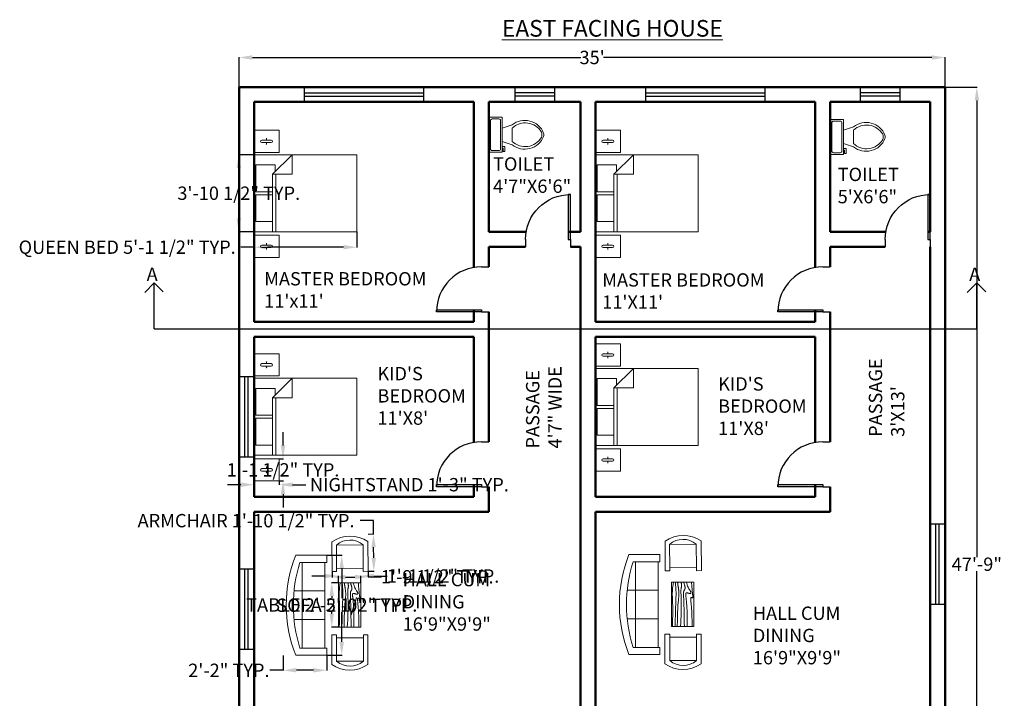
# Model space of a CAD drawing. Units: inches. Extents: x 179 to 2009, y 628 to 2084.
# Tile 4 of 5: x 635 to 1226, y 1676 to 2084. Entities that reach past the tile are written whole.
import ezdxf

# ---------------------------------------------------------------- set-up
doc = ezdxf.new("R2010")
doc.units = ezdxf.units.IN
doc.header["$MEASUREMENT"] = 0
for name, color, linetype, lineweight in [('A-ANNO-DIMS', 2, 'Continuous', 18), ('A-ANNO-SYMB', 5, 'Continuous', 25), ('A-ANNO-TEXT', 7, 'Continuous', 18), ('A-DOOR', 3, 'Continuous', 25), ('A-FURN', 4, 'Continuous', 18), ('A-GLAZ', 2, 'Continuous', 25), ('A-WALL', 1, 'Continuous', 50)]:
    doc.layers.add(name, color=color, linetype=linetype, lineweight=lineweight)
doc.styles.get("Standard").update_dxf_attribs({"font": 'arial.ttf'})
doc.dimstyles.get("Standard").update_dxf_attribs({"dimtxt": 8, "dimasz": 8, "dimexe": 0.18, "dimexo": 0.0625, "dimgap": 0.09, "dimtad": 0, "dimtih": 1, "dimtoh": 1, "dimdec": 0, "dimzin": 0, "dimdsep": 46, "dimlunit": 3, "dimtxsty": 'Standard', "dimcen": 0.09, "dimadec": 0, "dimazin": 0, "dimtfac": 1, "dimtdec": 0, "dimtofl": 0, "dimtmove": 0, "dimatfit": 3, "dimfxl": 1, "dimtolj": 1, "dimtzin": 0, "dimarcsym": 0})

# ---------------------------------------------------------------- blocks, each defined once
blk = doc.blocks.new('*U4')
for p, q in [((0, 0), (0, -6)), ((36, 0), (36, -6))]:
    blk.add_line(p, q)
blk.add_lwpolyline([(0, 0), (0, 36), (1.75, 36), (1.75, 0)], close=True)
blk.add_arc((0, 0), 36, 0, 90)
blk = doc.blocks.new('Bed - Queen')
for p, q in [((0, -80.00003), (0, 0)), ((0, 0), (59.99999, 0)), ((59.99999, 0), (59.99999, -80.00003)), ((7.99999, -1.2), (28.79998, -1.2)), ((7.99999, -14.4), (7.99999, -1.2)), ((28.79998, -1.2), (28.79998, -14.4)), ((31.19999, -1.2), (51.99999, -1.2)), ((31.19999, -14.4), (31.19999, -1.2)), ((51.99999, -1.2), (51.99999, -16.4)), ((0, -14.4), (44.8, -14.4)), ((59.99999, -29.6), (44.8, -14.4)), ((44.8, -14.4), (44.8, -29.6)), ((44.8, -16.8), (0, -16.8)), ((51.99999, -16.4), (46.79936, -16.4)), ((44.8, -29.6), (59.99999, -29.6)), ((59.99999, -80.00003), (0, -80.00003))]:
    blk.add_line(p, q)
blk = doc.blocks.new('*U3')
for p, q in [((9.5, -6), (9.5, -2)), ((-10, -8.5), (-8, -8.5)), ((-10, -9.5), (-10, -8.5)), ((-7, -9.5), (-10, -9.5)), ((-8, -8.5), (-8, -8)), ((-7, -8), (-7, -9.5)), ((-4, -8), (-6, -14)), ((4, -8), (6, -14)), ((4, -14), (-4, -14))]:
    blk.add_line(p, q)
blk.add_lwpolyline([(10.5, -8), (10.5, 0), (-10.5, 0), (-10.5, -8)], close=True)
for points in [[(-9.5, -2), (-9.5, -6)], [(8.5, -1), (-8.5, -1)], [(-8.5, -7), (8.5, -7)]]:
    blk.add_lwpolyline(points)
for centre, radius, start, end in [((-8.62, -1.88), 0.884, 81.8699, 188.1301), ((8.62, -1.88), 0.884, 351.8699, 98.1301), ((-8.62, -6.12), 0.884, 171.8699, 278.1301), ((8.62, -6.12), 0.884, 261.8699, 8.1301), ((3.52, -21.58), 12.17, 141.46911, 247.97143), ((4.2, -21.82), 11.33, 136.36773, 238.94682), ((-3.52, -21.58), 12.17, 292.02843, 38.53071), ((-4.2, -21.82), 11.33, 301.05301, 43.63209), ((0, -27.88), 4, 245.73182, 294.26817), ((0, -29), 4, 254.86053, 285.13947)]:
    blk.add_arc(centre, radius, start, end)
blk = doc.blocks.new('Sofa - Roundback 7 ft.')
for p, q in [((-12.00002, -32.4421), (-12.00003, -6.5971)), ((11.99997, -32.4421), (11.99998, -6.5971)), ((-36.000027, -34), (-36.000027, -11.4696)), ((-35.999844, -13.3819), (35.9998, -13.3819)), ((35.99998, -34), (35.99998, -11.4696)), ((-36.000027, -32.4421), (35.99998, -32.4421))]:
    blk.add_line(p, q)
for points in [[(-36.000027, -34), (-42.000027, -34), (-42.000027, -8)], [(41.99998, -8), (41.99998, -34), (35.99998, -34)]]:
    blk.add_lwpolyline(points)
for centre, radius, start, end in [((0, -114.25), 114.25, 68.43141, 111.5686), ((-0.00001, -127.1968), 121.1968, 72.72033, 107.2797)]:
    blk.add_arc(centre, radius, start, end)
blk = doc.blocks.new('Table - Rectangular Woodgrain 60 x 30 in.')
for p, q in [((0, 0), (0, -30)), ((60, 0), (0, 0)), ((60, -30), (60, 0)), ((0, -30), (60, -30))]:
    blk.add_line(p, q)
for points in [[(0, -2.4), (4.8155, -2.418), (9.0302, -2.4688), (12.709, -2.5477), (15.9167, -2.65), (18.7181, -2.7711), (21.1781, -2.9063), (23.3616, -3.0508), (25.3333, -3.2), (27.1477, -3.3495), (28.8172, -3.4958), (30.3437, -3.636), (31.7291, -3.7667), (32.9756, -3.8849), (34.0849, -3.9875), (35.059, -4.0714), (35.9, -4.1334), (36.6114, -4.1711), (37.2041, -4.1854), (37.6906, -4.1779), (38.0833, -4.15), (38.3948, -4.1034), (38.6375, -4.0396), (38.8239, -3.9602), (38.9666, -3.8667), (39.0764, -3.7608), (39.1573, -3.6448), (39.2116, -3.521), (39.2416, -3.3917), (39.2498, -3.2593), (39.2385, -3.1261), (39.21, -2.9944), (39.1666, -2.8667), (39.111, -2.7447), (39.0468, -2.6281), (38.978, -2.5163), (38.9083, -2.4083), (38.8418, -2.3035), (38.7823, -2.201), (38.7337, -2.1001), (38.7, -2), (38.6844, -1.9003), (38.6875, -1.8021), (38.7094, -1.707), (38.75, -1.6167), (38.8094, -1.5326), (38.8875, -1.4563), (38.9844, -1.3893), (39.1, -1.3333), (39.2351, -1.2896), (39.3937, -1.2583), (39.5804, -1.2396), (39.8, -1.2333), (40.057, -1.2396), (40.3562, -1.2583), (40.7023, -1.2896), (41.1, -1.3333), (41.5547, -1.3895), (42.0755, -1.4573), (42.6721, -1.5361), (43.3542, -1.625), (44.1316, -1.7233), (45.014, -1.8302), (46.0114, -1.9449), (47.1333, -2.0667), (48.3862, -2.1947), (49.7625, -2.3281), (51.2513, -2.4663), (52.8416, -2.6083), (54.5226, -2.7535), (56.2833, -2.9011), (58.1127, -3.0501), (60, -3.2)], [(0, -9.2), (6.5759, -9.0858), (11.9385, -9.0365), (16.2527, -9.0418), (19.6833, -9.0917), (22.3952, -9.1759), (24.5531, -9.2844), (26.322, -9.4069), (27.8666, -9.5333), (29.3241, -9.6553), (30.7203, -9.7719), (32.0532, -9.8837), (33.3208, -9.9917), (34.5213, -10.0965), (35.6526, -10.199), (36.7128, -10.2999), (37.7, -10.4), (38.6129, -10.4996), (39.4531, -10.5969), (40.223, -10.6895), (40.925, -10.775), (41.5613, -10.8512), (42.1344, -10.9156), (42.6465, -10.966), (43.1, -11), (43.4976, -11.0158), (43.8437, -11.0136), (44.143, -10.9942), (44.4, -10.9583), (44.6195, -10.9069), (44.8062, -10.8406), (44.9648, -10.7603), (45.1, -10.6667), (45.2155, -10.5598), (45.3114, -10.4365), (45.3871, -10.2929), (45.4416, -10.125), (45.4743, -9.929), (45.4844, -9.7011), (45.4709, -9.4371), (45.4333, -9.1333), (45.3716, -8.7883), (45.2896, -8.4104), (45.1919, -8.0107), (45.0833, -7.6), (44.9685, -7.1893), (44.8521, -6.7896), (44.7388, -6.4117), (44.6333, -6.0667), (44.54, -5.7628), (44.4614, -5.4979), (44.4001, -5.2675), (44.3583, -5.0667), (44.3384, -4.8909), (44.3427, -4.7354), (44.3736, -4.5956), (44.4333, -4.4667), (44.5236, -4.3453), (44.6427, -4.2333), (44.7884, -4.1339), (44.9583, -4.05), (45.1501, -3.9849), (45.3614, -3.9417), (45.59, -3.9234), (45.8333, -3.9333), (46.0915, -3.9749), (46.3734, -4.0531), (46.6906, -4.1736), (47.0542, -4.3417), (47.4756, -4.5629), (47.9661, -4.8427), (48.5372, -5.1866), (49.2, -5.6), (49.9676, -6.0844), (50.8594, -6.625), (51.8965, -7.2031), (53.1, -7.8), (54.491, -8.3969), (56.0906, -8.975), (57.9199, -9.5156), (60, -10)], [(0, -12.8), (5.1847, -12.9322), (9.6213, -13.0323), (13.3963, -13.1059), (16.5958, -13.1583), (19.3063, -13.1952), (21.614, -13.2219), (23.6054, -13.2439), (25.3666, -13.2667), (26.9728, -13.2947), (28.4531, -13.3281), (29.8256, -13.3663), (31.1083, -13.4083), (32.3191, -13.4535), (33.476, -13.501), (34.597, -13.5501), (35.7, -13.6), (36.7984, -13.6497), (37.8875, -13.6979), (38.9578, -13.743), (40, -13.7833), (41.0047, -13.8174), (41.9625, -13.8438), (42.864, -13.8607), (43.7, -13.8667), (44.4631, -13.8604), (45.1552, -13.8417), (45.7801, -13.8104), (46.3416, -13.7667), (46.8439, -13.7104), (47.2906, -13.6417), (47.6858, -13.5604), (48.0333, -13.4667), (48.3375, -13.3608), (48.6042, -13.2448), (48.8396, -13.121), (49.05, -12.9917), (49.2417, -12.8593), (49.4208, -12.7261), (49.5937, -12.5944), (49.7667, -12.4667), (49.9452, -12.3451), (50.1323, -12.2313), (50.3303, -12.1268), (50.5416, -12.0333), (50.7686, -11.9524), (51.0135, -11.8854), (51.2788, -11.8341), (51.5666, -11.8), (51.8785, -11.7843), (52.2116, -11.7865), (52.562, -11.8059), (52.926, -11.8417), (53.2998, -11.8931), (53.6795, -11.9594), (54.0614, -12.0397), (54.4416, -12.1333), (54.8223, -12.2401), (55.2293, -12.3625), (55.6942, -12.5037), (56.2489, -12.6667), (56.9251, -12.8547), (57.7545, -13.0708), (58.7689, -13.3182), (60, -13.6)], [(0, -18), (5.124, -17.7273), (9.6609, -17.5057), (13.6705, -17.3303), (17.2125, -17.1958), (20.3467, -17.0973), (23.1328, -17.0297), (25.6307, -16.9878), (27.9, -16.9667), (29.9928, -16.9617), (31.9302, -16.9703), (33.7254, -16.9907), (35.3917, -17.0208), (36.9423, -17.0588), (38.3906, -17.1026), (39.7499, -17.1503), (41.0333, -17.2), (42.2519, -17.2496), (43.4073, -17.2969), (44.4986, -17.3395), (45.525, -17.375), (46.4858, -17.4012), (47.3802, -17.4156), (48.2074, -17.416), (48.9667, -17.4), (49.6583, -17.3662), (50.2872, -17.3167), (50.8595, -17.2547), (51.3812, -17.1833), (51.8584, -17.1057), (52.2971, -17.025), (52.7034, -16.9443), (53.0833, -16.8667), (53.443, -16.7951), (53.789, -16.7313), (54.128, -16.6768), (54.4666, -16.6334), (54.8115, -16.6024), (55.1693, -16.5854), (55.5465, -16.5841), (55.95, -16.6), (56.3828, -16.6337), (56.8346, -16.6823), (57.2915, -16.7418), (57.7396, -16.8084), (58.165, -16.878), (58.5539, -16.9469), (58.8924, -17.0111), (59.1666, -17.0667), (59.3679, -17.1107), (59.5078, -17.1438), (59.6032, -17.1675), (59.6708, -17.1833), (59.7275, -17.193), (59.7901, -17.1979), (59.8753, -17.1998), (60, -17.2)], [(0, -22.4), (8.0098, -22.2501), (14.4094, -22.1011), (19.4168, -21.9535), (23.25, -21.8083), (26.1269, -21.6663), (28.2656, -21.5281), (29.884, -21.3947), (31.2, -21.2667), (32.3967, -21.1448), (33.5172, -21.0292), (34.5697, -20.9198), (35.5625, -20.8167), (36.5037, -20.7198), (37.4015, -20.6292), (38.2642, -20.5448), (39.1, -20.4667), (39.9164, -20.3951), (40.7187, -20.3313), (41.5117, -20.2768), (42.3, -20.2333), (43.0883, -20.2024), (43.8812, -20.1854), (44.6836, -20.1841), (45.5, -20.2), (46.3328, -20.234), (47.1747, -20.2844), (48.0163, -20.3488), (48.8479, -20.425), (49.66, -20.5106), (50.4429, -20.6031), (51.1872, -20.7004), (51.8833, -20.8), (52.5246, -20.8999), (53.1166, -20.9995), (53.6681, -21.0983), (54.1875, -21.1958), (54.6834, -21.2919), (55.1646, -21.3859), (55.6394, -21.4777), (56.1167, -21.5667), (56.6028, -21.6515), (57.0961, -21.7266), (57.5929, -21.7852), (58.0896, -21.8208), (58.5823, -21.8268), (59.0674, -21.7964), (59.5412, -21.723), (60, -21.6)], [(0, -25.2), (8.6355, -25.0504), (15.7026, -24.9031), (21.4049, -24.7606), (25.9458, -24.625), (29.529, -24.4988), (32.3578, -24.3844), (34.6359, -24.284), (36.5667, -24.2), (38.3213, -24.1341), (39.9417, -24.0854), (41.437, -24.0523), (42.8167, -24.0333), (44.0901, -24.0268), (45.2667, -24.0313), (46.3557, -24.0451), (47.3667, -24.0667), (48.309, -24.0947), (49.1928, -24.1287), (50.0284, -24.168), (50.826, -24.2125), (51.5959, -24.2617), (52.3483, -24.3151), (53.0935, -24.3725), (53.8417, -24.4334), (54.6009, -24.497), (55.3699, -24.561), (56.1454, -24.6226), (56.9239, -24.6792), (57.7021, -24.7279), (58.4764, -24.7662), (59.2435, -24.7911), (60, -24.8)], [(0, -28.8), (5.6867, -28.6681), (10.45, -28.5698), (14.407, -28.5012), (17.675, -28.4584), (20.3711, -28.4374), (22.6125, -28.4344), (24.5164, -28.4455), (26.2, -28.4667), (27.762, -28.4947), (29.2276, -28.5281), (30.6033, -28.5663), (31.8958, -28.6084), (33.1118, -28.6535), (34.2578, -28.7011), (35.3405, -28.7501), (36.3666, -28.8), (37.3443, -28.8497), (38.288, -28.8974), (39.2137, -28.9412), (40.1375, -28.9792), (41.0753, -29.0093), (42.0432, -29.0297), (43.0572, -29.0384), (44.1333, -29.0333), (45.2936, -29.0114), (46.5843, -28.9641), (48.0579, -28.8816), (49.7666, -28.7542), (51.7629, -28.5721), (54.0989, -28.3255), (56.8272, -28.0048), (60, -27.6)]]:
    blk.add_lwpolyline(points)
blk = doc.blocks.new('*D17')
at = {"layer": 'A-ANNO-DIMS', "color": 0, "lineweight": -2, "transparency": 16777216}
for p, q in [((766.49, 2043.24), (766.49, 2061.08)), ((774.49, 2060.9), (971.62, 2060.9)), ((1182.49, 2060.9), (985.37, 2060.9)), ((1190.49, 2043.24), (1190.49, 2061.08))]:
    blk.add_line(p, q, dxfattribs=at)
at = {"layer": 'A-ANNO-DIMS', "color": 0, "transparency": 16777216}
for points in [[(774.49, 2062.23), (774.49, 2059.56), (766.49, 2060.9)], [(1182.49, 2062.23), (1182.49, 2059.56), (1190.49, 2060.9)]]:
    blk.add_solid(points, dxfattribs=at)
at = {"layer": 'Defpoints', "color": 0, "transparency": 16777216}
for p in [(1190.49, 2060.9), (766.49, 2043.18), (1190.49, 2043.18)]:
    blk.add_point(p, dxfattribs=at)
at = {"layer": 'A-ANNO-DIMS', "color": 0, "transparency": 16777216, "insert": (978.49, 2060.9), "char_height": 8, "attachment_point": 5}
blk.add_mtext("\\A1;35'", dxfattribs=at)
blk = doc.blocks.new('*D18')
at = {"layer": 'A-ANNO-DIMS', "color": 0, "lineweight": -2, "transparency": 16777216}
for p, q in [((1190.56, 2043.18), (1209.72, 2043.18)), ((1209.54, 2035.18), (1209.54, 1760.86)), ((1209.54, 1478.18), (1209.54, 1752.51)), ((1190.56, 1470.18), (1209.72, 1470.18))]:
    blk.add_line(p, q, dxfattribs=at)
at = {"layer": 'A-ANNO-DIMS', "color": 0, "transparency": 16777216}
for points in [[(1208.21, 2035.18), (1210.88, 2035.18), (1209.54, 2043.18)], [(1208.21, 1478.18), (1210.88, 1478.18), (1209.54, 1470.18)]]:
    blk.add_solid(points, dxfattribs=at)
at = {"layer": 'Defpoints', "color": 0, "transparency": 16777216}
for p in [(1190.49, 2043.18), (1190.49, 1470.18), (1209.54, 1470.18)]:
    blk.add_point(p, dxfattribs=at)
at = {"layer": 'A-ANNO-DIMS', "color": 0, "transparency": 16777216, "insert": (1209.54, 1756.68), "char_height": 8, "attachment_point": 5}
blk.add_mtext('\\A1;47\'-9"', dxfattribs=at)
blk = doc.blocks.new('ARMCHAIR')
for p, q in [((0, 0), (0, 17.87)), ((21.68, 0), (21.68, 17.87)), ((2.68, 1.83), (2.68, 15.94)), ((2.68, 15.94), (18.72, 15.94)), ((18.72, 15.94), (18.72, 1.83)), ((2.68, 0), (0, 0)), ((18.72, 1.83), (2.68, 1.83)), ((2.68, 1.83), (2.68, 0)), ((18.72, 1.83), (18.72, 0)), ((18.72, 0), (21.68, 0))]:
    blk.add_line(p, q)
for centre, radius, start, end in [((10.84, 2.23), 19.03, 55.27776, 124.72224), ((10.7, 6.48), 12.4, 49.71958, 130.28042)]:
    blk.add_arc(centre, radius, start, end)
blk = doc.blocks.new('NIGHTSTAND')
for p, q in [((4.59, 7.37), (10.22, 7.37)), ((7.41, 8.38), (7.27, 8.28)), ((7.41, 7.37), (7.41, 8.38)), ((7.41, 8.38), (7.55, 8.28)), ((4.59, 5.83), (10.22, 5.83)), ((7.41, 4.88), (7.23, 5.01)), ((7.41, 5.83), (7.41, 4.88)), ((7.41, 4.88), (7.58, 5))]:
    blk.add_line(p, q)
blk.add_lwpolyline([(0, 13.3), (15.09, 13.3), (15.09, 0), (0, 0)], close=True)
for centre, start, end in [((4.59, 6.6), 90, 270), ((10.22, 6.6), 270, 90)]:
    blk.add_arc(centre, 0.771, start, end)
blk = doc.blocks.new('*D45')
at = {"layer": 'A-ANNO-DIMS', "color": 0, "lineweight": -2, "transparency": 16777216}
for p, q in [((775.49, 1956.21), (775.49, 1946.84)), ((837.19, 1956.21), (837.19, 1946.84)), ((775.49, 1947.02), (767.49, 1947.02)), ((829.19, 1947.02), (783.49, 1947.02))]:
    blk.add_line(p, q, dxfattribs=at)
at = {"layer": 'A-ANNO-DIMS', "color": 0, "transparency": 16777216}
for points in [[(783.49, 1948.35), (783.49, 1945.69), (775.49, 1947.02)], [(829.19, 1948.35), (829.19, 1945.69), (837.19, 1947.02)]]:
    blk.add_solid(points, dxfattribs=at)
at = {"layer": 'Defpoints', "color": 0, "transparency": 16777216}
for p in [(775.49, 1956.28), (837.19, 1956.28), (775.49, 1947.02)]:
    blk.add_point(p, dxfattribs=at)
at = {"layer": 'A-ANNO-DIMS', "color": 0, "transparency": 16777216, "insert": (699.24, 1947.02), "char_height": 8, "attachment_point": 5}
blk.add_mtext('\\A1;QUEEN BED 5\'-1 1/2" TYP.', dxfattribs=at)
blk = doc.blocks.new('*D46')
at = {"layer": 'A-ANNO-DIMS', "color": 0, "lineweight": -2, "transparency": 16777216}
for p, q in [((775.43, 2002.55), (766.06, 2002.55)), ((766.24, 1994.55), (766.24, 1983.64)), ((766.24, 1964.28), (766.24, 1975.18)), ((775.43, 1956.28), (766.06, 1956.28))]:
    blk.add_line(p, q, dxfattribs=at)
at = {"layer": 'A-ANNO-DIMS', "color": 0, "transparency": 16777216}
for points in [[(764.91, 1994.55), (767.57, 1994.55), (766.24, 2002.55)], [(764.91, 1964.28), (767.57, 1964.28), (766.24, 1956.28)]]:
    blk.add_solid(points, dxfattribs=at)
at = {"layer": 'Defpoints', "color": 0, "transparency": 16777216}
for p in [(766.24, 2002.55), (775.49, 2002.55), (775.49, 1956.28)]:
    blk.add_point(p, dxfattribs=at)
at = {"layer": 'A-ANNO-DIMS', "color": 0, "transparency": 16777216, "insert": (766.24, 1979.41), "char_height": 8, "attachment_point": 5}
blk.add_mtext('\\A1;3\'-10 1/2" TYP.', dxfattribs=at)
blk = doc.blocks.new('*D47')
at = {"layer": 'A-ANNO-DIMS', "color": 0, "lineweight": -2, "transparency": 16777216}
for p, q in [((767.49, 1804.42), (759.49, 1804.42)), ((775.49, 1806.62), (775.49, 1804.24)), ((790.58, 1806.62), (790.58, 1804.24)), ((798.58, 1804.42), (806.58, 1804.42))]:
    blk.add_line(p, q, dxfattribs=at)
at = {"layer": 'A-ANNO-DIMS', "color": 0, "transparency": 16777216}
for points in [[(767.49, 1805.75), (767.49, 1803.08), (775.49, 1804.42)], [(798.58, 1805.75), (798.58, 1803.08), (790.58, 1804.42)]]:
    blk.add_solid(points, dxfattribs=at)
at = {"layer": 'Defpoints', "color": 0, "transparency": 16777216}
for p in [(775.49, 1806.68), (790.58, 1806.68), (790.58, 1804.42)]:
    blk.add_point(p, dxfattribs=at)
at = {"layer": 'A-ANNO-DIMS', "color": 0, "transparency": 16777216, "insert": (868.73, 1804.42), "char_height": 8, "attachment_point": 5}
blk.add_mtext('\\A1;NIGHTSTAND 1\'-3" TYP.', dxfattribs=at)
blk = doc.blocks.new('*D48')
at = {"layer": 'A-ANNO-DIMS', "color": 0, "lineweight": -2, "transparency": 16777216}
for p, q in [((792.85, 1827.98), (792.85, 1835.98)), ((790.64, 1819.98), (793.03, 1819.98)), ((790.64, 1806.68), (793.03, 1806.68)), ((792.85, 1798.68), (792.85, 1790.68))]:
    blk.add_line(p, q, dxfattribs=at)
at = {"layer": 'A-ANNO-DIMS', "color": 0, "transparency": 16777216}
for points in [[(791.51, 1827.98), (794.18, 1827.98), (792.85, 1819.98)], [(791.51, 1798.68), (794.18, 1798.68), (792.85, 1806.68)]]:
    blk.add_solid(points, dxfattribs=at)
at = {"layer": 'Defpoints', "color": 0, "transparency": 16777216}
for p in [(790.58, 1819.98), (792.85, 1819.98), (790.58, 1806.68)]:
    blk.add_point(p, dxfattribs=at)
at = {"layer": 'A-ANNO-DIMS', "color": 0, "transparency": 16777216, "insert": (792.85, 1813.33), "char_height": 8, "attachment_point": 5}
blk.add_mtext('\\A1;1\'-1 1/2" TYP.', dxfattribs=at)
blk = doc.blocks.new('*D51')
at = {"layer": 'A-ANNO-DIMS', "color": 0, "lineweight": -2, "transparency": 16777216}
for p, q in [((847.11, 1782.83), (839.11, 1782.83)), ((847.18, 1774.83), (847.11, 1782.83)), ((843.89, 1774.8), (847.36, 1774.83)), ((847.3, 1760.44), (847.25, 1766.83)), ((844.07, 1752.41), (847.55, 1752.44))]:
    blk.add_line(p, q, dxfattribs=at)
at = {"layer": 'A-ANNO-DIMS', "color": 0, "transparency": 16777216}
for points in [[(848.58, 1766.84), (845.92, 1766.82), (847.18, 1774.83)], [(848.64, 1760.45), (845.97, 1760.43), (847.37, 1752.44)]]:
    blk.add_solid(points, dxfattribs=at)
at = {"layer": 'Defpoints', "color": 0, "transparency": 16777216}
for p in [(843.82, 1774.8), (847.18, 1774.83), (844.01, 1752.41)]:
    blk.add_point(p, dxfattribs=at)
at = {"layer": 'A-ANNO-DIMS', "color": 0, "transparency": 16777216, "insert": (770.63, 1782.83), "char_height": 8, "attachment_point": 5}
blk.add_mtext('\\A1;ARMCHAIR 1\'-10 1/2" TYP.', dxfattribs=at)
blk = doc.blocks.new('*D52')
at = {"layer": 'A-ANNO-DIMS', "color": 0, "lineweight": -2, "transparency": 16777216}
for p, q in [((822.33, 1752.17), (822.36, 1748.69)), ((844.01, 1752.35), (844.04, 1748.87)), ((830.36, 1748.94), (836.04, 1748.99)), ((844.04, 1749.05), (852.04, 1749.12))]:
    blk.add_line(p, q, dxfattribs=at)
at = {"layer": 'A-ANNO-DIMS', "color": 0, "transparency": 16777216}
for points in [[(830.35, 1750.27), (830.37, 1747.6), (822.36, 1748.87)], [(836.03, 1750.32), (836.05, 1747.65), (844.04, 1749.05)]]:
    blk.add_solid(points, dxfattribs=at)
at = {"layer": 'Defpoints', "color": 0, "transparency": 16777216}
for p in [(822.33, 1752.23), (844.01, 1752.41), (844.04, 1749.05)]:
    blk.add_point(p, dxfattribs=at)
at = {"layer": 'A-ANNO-DIMS', "color": 0, "transparency": 16777216, "insert": (885.46, 1749.12), "char_height": 8, "attachment_point": 5}
blk.add_mtext('\\A1;1\'-9 1/2" TYP.', dxfattribs=at)
blk = doc.blocks.new('*D57')
at = {"layer": 'A-ANNO-DIMS', "color": 0, "lineweight": -2, "transparency": 16777216}
for p, q in [((819.14, 1762.08), (828.27, 1762.08)), ((828.09, 1754.08), (828.09, 1736.26)), ((828.09, 1710), (828.09, 1727.81)), ((819.14, 1702), (828.27, 1702))]:
    blk.add_line(p, q, dxfattribs=at)
at = {"layer": 'A-ANNO-DIMS', "color": 0, "transparency": 16777216}
for points in [[(826.76, 1754.08), (829.42, 1754.08), (828.09, 1762.08)], [(826.76, 1710), (829.42, 1710), (828.09, 1702)]]:
    blk.add_solid(points, dxfattribs=at)
at = {"layer": 'Defpoints', "color": 0, "transparency": 16777216}
for p in [(819.08, 1762.08), (819.08, 1702), (828.09, 1702)]:
    blk.add_point(p, dxfattribs=at)
at = {"layer": 'A-ANNO-DIMS', "color": 0, "transparency": 16777216, "insert": (828.09, 1732.04), "char_height": 8, "attachment_point": 5}
blk.add_mtext('\\A1;SOFA 5\'-0" TYP.', dxfattribs=at)
blk = doc.blocks.new('*D58')
at = {"layer": 'A-ANNO-DIMS', "color": 0, "lineweight": -2, "transparency": 16777216}
for p, q in [((792.85, 1701.93), (792.85, 1692.8)), ((819.08, 1701.93), (819.08, 1692.8)), ((792.85, 1692.98), (784.85, 1692.98)), ((811.08, 1692.98), (800.85, 1692.98))]:
    blk.add_line(p, q, dxfattribs=at)
at = {"layer": 'A-ANNO-DIMS', "color": 0, "transparency": 16777216}
for points in [[(800.85, 1694.32), (800.85, 1691.65), (792.85, 1692.98)], [(811.08, 1694.32), (811.08, 1691.65), (819.08, 1692.98)]]:
    blk.add_solid(points, dxfattribs=at)
at = {"layer": 'Defpoints', "color": 0, "transparency": 16777216}
for p in [(792.85, 1702), (819.08, 1702), (792.85, 1692.98)]:
    blk.add_point(p, dxfattribs=at)
at = {"layer": 'A-ANNO-DIMS', "color": 0, "transparency": 16777216, "insert": (760.31, 1692.98), "char_height": 8, "attachment_point": 5}
blk.add_mtext('\\A1;2\'-2" TYP.', dxfattribs=at)
blk = doc.blocks.new('*D59')
at = {"layer": 'A-ANNO-DIMS', "color": 0, "lineweight": -2, "transparency": 16777216}
for p, q in [((826.05, 1745.58), (821.92, 1745.58)), ((822.1, 1737.58), (822.1, 1736.44)), ((822.1, 1726.84), (822.1, 1727.98)), ((826.05, 1718.84), (821.92, 1718.84))]:
    blk.add_line(p, q, dxfattribs=at)
at = {"layer": 'A-ANNO-DIMS', "color": 0, "transparency": 16777216}
for points in [[(820.76, 1737.58), (823.43, 1737.58), (822.1, 1745.58)], [(820.76, 1726.84), (823.43, 1726.84), (822.1, 1718.84)]]:
    blk.add_solid(points, dxfattribs=at)
at = {"layer": 'Defpoints', "color": 0, "transparency": 16777216}
for p in [(822.1, 1745.58), (826.11, 1745.58), (826.11, 1718.84)]:
    blk.add_point(p, dxfattribs=at)
at = {"layer": 'A-ANNO-DIMS', "color": 0, "transparency": 16777216, "insert": (822.1, 1732.21), "char_height": 8, "attachment_point": 5}
blk.add_mtext('\\A1;TABLE 2\'-2 1/2" TYP.', dxfattribs=at)
blk = doc.blocks.new('*D60')
at = {"layer": 'A-ANNO-DIMS', "color": 0, "lineweight": -2, "transparency": 16777216}
for p, q in [((818.11, 1749.59), (810.11, 1749.59)), ((826.11, 1745.64), (826.11, 1749.77)), ((839.48, 1745.64), (839.48, 1749.77)), ((847.48, 1749.59), (855.48, 1749.59))]:
    blk.add_line(p, q, dxfattribs=at)
at = {"layer": 'A-ANNO-DIMS', "color": 0, "transparency": 16777216}
for points in [[(818.11, 1750.93), (818.11, 1748.26), (826.11, 1749.59)], [(847.48, 1750.93), (847.48, 1748.26), (839.48, 1749.59)]]:
    blk.add_solid(points, dxfattribs=at)
at = {"layer": 'Defpoints', "color": 0, "transparency": 16777216}
for p in [(826.11, 1745.58), (839.48, 1749.59), (839.48, 1745.58)]:
    blk.add_point(p, dxfattribs=at)
at = {"layer": 'A-ANNO-DIMS', "color": 0, "transparency": 16777216, "insert": (888.9, 1749.59), "char_height": 8, "attachment_point": 5}
blk.add_mtext('\\A1;1\'-1 1/2" TYP.', dxfattribs=at)

msp = doc.modelspace()

# ---------------------------------------------------------------- linework, layer by layer
at = {"layer": 'A-ANNO-SYMB'}
for p, q in [((715.52, 1925.56), (709.76, 1919.84)), ((715.52, 1898.02), (715.52, 1925.56)), ((715.52, 1925.56), (720.84, 1920.21)), ((1209.54, 1925.56), (1203.79, 1919.84)), ((1209.54, 1898.02), (1209.54, 1925.56)), ((1209.54, 1925.56), (1214.86, 1920.21)), ((715.52, 1898.02), (1209.54, 1898.02))]:
    msp.add_line(p, q, dxfattribs=at)
at = {"layer": 'A-GLAZ'}
for p, q in [((805.49, 2039.68), (877.49, 2039.68)), ((805.49, 2037.68), (877.49, 2037.68)), ((955.99, 2039.68), (931.99, 2039.68)), ((955.99, 2037.68), (931.99, 2037.68)), ((1010.49, 2039.68), (1082.49, 2039.68)), ((1010.49, 2037.68), (1082.49, 2037.68)), ((1163.49, 2039.68), (1139.49, 2039.68)), ((1163.49, 2037.68), (1139.49, 2037.68)), ((769.99, 1821.18), (769.99, 1869.18)), ((771.99, 1821.18), (771.99, 1869.18)), ((1184.99, 1732.68), (1184.99, 1780.68)), ((1186.99, 1732.68), (1186.99, 1780.68)), ((769.99, 1705.68), (769.99, 1753.68)), ((771.99, 1705.68), (771.99, 1753.68))]:
    msp.add_line(p, q, dxfattribs=at)
for points in [[(805.49, 2034.18), (877.49, 2034.18), (877.49, 2043.18), (805.49, 2043.18)], [(955.99, 2043.18), (931.99, 2043.18), (931.99, 2034.18), (955.99, 2034.18)], [(1010.49, 2034.18), (1082.49, 2034.18), (1082.49, 2043.18), (1010.49, 2043.18)], [(1163.49, 2043.18), (1139.49, 2043.18), (1139.49, 2034.18), (1163.49, 2034.18)], [(775.49, 1821.18), (775.49, 1869.18), (766.49, 1869.18), (766.49, 1821.18)], [(1190.49, 1732.68), (1190.49, 1780.68), (1181.49, 1780.68), (1181.49, 1732.68)], [(775.49, 1705.68), (775.49, 1753.68), (766.49, 1753.68), (766.49, 1705.68)]]:
    msp.add_lwpolyline(points, close=True, dxfattribs=at)
at = {"layer": 'A-WALL'}
for p, q in [((766.49, 2043.18), (1190.49, 2043.18)), ((766.49, 2043.18), (766.49, 1470.18)), ((1190.49, 2043.18), (1190.49, 1470.18)), ((775.49, 2034.18), (907.49, 2034.18)), ((775.49, 2034.18), (775.49, 1902.18)), ((907.49, 2034.18), (907.49, 1934.8)), ((916.49, 2034.18), (916.49, 1956.18)), ((916.49, 2034.18), (971.49, 2034.18)), ((971.49, 2034.18), (971.49, 1956.18)), ((980.49, 2034.18), (980.49, 1902.18)), ((980.49, 2034.18), (1112.49, 2034.18)), ((1112.49, 2034.18), (1112.49, 1934.8)), ((1121.49, 2034.18), (1121.49, 1956.18)), ((1121.49, 2034.18), (1181.49, 2034.18)), ((1181.49, 2034.18), (1181.49, 1956.18)), ((916.49, 1956.18), (938.87, 1956.18)), ((964.18, 1956.18), (971.49, 1956.18)), ((1121.49, 1956.18), (1154.87, 1956.18)), ((1180.18, 1956.18), (1181.49, 1956.18)), ((916.49, 1947.18), (938.49, 1947.18)), ((916.49, 1947.18), (916.49, 1935.18)), ((965.49, 1947.18), (971.49, 1947.18)), ((971.49, 1947.18), (971.49, 1566.18)), ((1121.49, 1947.18), (1154.49, 1947.18)), ((1121.49, 1947.18), (1121.49, 1935.18)), ((1181.49, 1947.18), (1181.49, 1566.18)), ((907.49, 1909.49), (907.49, 1902.18)), ((916.49, 1908.18), (916.49, 1830.18)), ((1112.49, 1909.49), (1112.49, 1902.18)), ((1121.49, 1908.18), (1121.49, 1830.13)), ((775.49, 1902.18), (907.49, 1902.18)), ((980.49, 1902.18), (1112.49, 1902.18)), ((775.49, 1893.18), (907.49, 1893.18)), ((775.49, 1893.18), (775.49, 1797.18)), ((907.49, 1893.18), (907.49, 1829.8)), ((980.49, 1893.18), (1112.49, 1893.18)), ((980.49, 1893.18), (980.49, 1797.18)), ((1112.49, 1893.18), (1112.49, 1829.75)), ((907.49, 1804.49), (907.49, 1797.18)), ((1112.49, 1804.44), (1112.49, 1797.18)), ((916.49, 1803.18), (916.49, 1788.18)), ((1121.49, 1803.13), (1121.49, 1788.18)), ((775.49, 1797.18), (907.49, 1797.18)), ((980.49, 1797.18), (1112.49, 1797.18)), ((775.49, 1788.18), (916.49, 1788.18)), ((775.49, 1788.18), (775.49, 1671.18)), ((980.49, 1788.18), (1121.49, 1788.18)), ((980.49, 1788.18), (980.49, 1671.18))]:
    msp.add_line(p, q, dxfattribs=at)

# ---------------------------------------------------------------- block references
at = {"layer": 'A-DOOR', "xscale": -0.75, "yscale": 0.75, "zscale": 0.75}
for p in [(965.49, 1951.68), (1181.49, 1951.68)]:
    msp.add_blockref('*U4', p, dxfattribs=at)
at = {"layer": 'A-DOOR', "xscale": 0.75, "yscale": 0.75, "zscale": 0.75, "rotation": 90}
for p in [(911.99, 1908.18), (1116.99, 1908.18), (911.99, 1803.18), (1116.99, 1803.13)]:
    msp.add_blockref('*U4', p, dxfattribs=at)
at = {"layer": 'A-FURN'}
for name, p, rotation in [('*U3', (916.49, 2014.51), 90), ('*U3', (1121.49, 2013.24), 90), ('ARMCHAIR', (822.33, 1752.23), 0.4840249387552889), ('ARMCHAIR', (1022.44, 1752.62), 0.4840249387552889), ('ARMCHAIR', (843.77, 1714.36), 180), ('ARMCHAIR', (1043.87, 1714.75), 180)]:
    msp.add_blockref(name, p, dxfattribs=dict(at, rotation=rotation))
for p in [(775.49, 2003.96), (980.49, 2003.96), (775.49, 1940.91), (980.49, 1940.91), (980.49, 1875.67), (775.49, 1869.73), (980.49, 1812.62), (775.49, 1806.68)]:
    msp.add_blockref('NIGHTSTAND', p, dxfattribs=at)
for name, p, xscale, yscale, zscale, rotation in [('Bed - Queen', (775.49, 1956.28), 0.7711811969898703, 0.7711811969898703, 0.7711811969898703, 90), ('Bed - Queen', (980.49, 1956.28), 0.7711811969898703, 0.7711811969898703, 0.7711811969898703, 90), ('Bed - Queen', (980.49, 1827.99), 0.7711811969898703, 0.7711811969898703, 0.7711811969898703, 90), ('Bed - Queen', (775.49, 1822.05), 0.7711811969898703, 0.7711811969898703, 0.7711811969898703, 90), ('Sofa - Roundback 7 ft.', (994.86, 1732.43), -0.7152482803123178, 0.7152482803123178, 0.7152482803123178, 90), ('Sofa - Roundback 7 ft.', (794.76, 1732.04), -0.7152482803123178, 0.7152482803123178, 0.7152482803123178, 90), ('Table - Rectangular Woodgrain 60 x 30 in.', (839.48, 1718.84), -0.4457008028405438, 0.4457008028405438, 0.4457008028405438, 270), ('Table - Rectangular Woodgrain 60 x 30 in.', (1039.58, 1719.23), -0.4457008028405438, 0.4457008028405438, 0.4457008028405438, 270)]:
    msp.add_blockref(name, p, dxfattribs=dict(at, xscale=xscale, yscale=yscale, zscale=zscale, rotation=rotation))

# ---------------------------------------------------------------- texts
at = {"layer": 'A-ANNO-SYMB', "char_height": 8, "attachment_point": 1}
for insert in [(710.92, 1934.77), (1204.95, 1934.77)]:
    msp.add_mtext_dynamic_manual_height_columns('A', width=27.9691, gutter_width=1, heights=[0], dxfattribs=dict(at, insert=insert))
at = {"layer": 'A-ANNO-TEXT', "attachment_point": 1}
for s, width, heights, insert, char_height in [('{\\fArial|b1|i0|c0|p34;\\LEAST FACING HOUSE}', 293.7901, [0], (924.34, 2083.41), 10), ('TOILET\\P4\'7"X6\'6"', 129.4382, [0], (919, 2000.96), 8), ('TOILET\\P5\'X6\'6"', 129.4382, [0], (1125.97, 1994.7), 8), ("MASTER BEDROOM\\P11'x11'", 129.4382, [0], (781.53, 1932.04), 8), ("MASTER BEDROOM\\P11'X11'", 129.4382, [0], (984.55, 1931.35), 8), ("KID'S\\PBEDROOM\\P11'X8'", 129.4382, [0], (849.52, 1875.1), 8), ("KID'S \\PBEDROOM\\P11'X8'", 129.4382, [0], (1054.17, 1868.92), 8), ('HALL CUM\\PDINING\\P16\'9"X9\'9"', 129.4382, [0], (864.69, 1751.44), 8), ('HALL CUM\\PDINING\\P16\'9"X9\'9"', 129.4382, [56.89], (1074.99, 1731.24), 8)]:
    msp.add_mtext_dynamic_manual_height_columns(s, width=width, gutter_width=1, heights=heights, dxfattribs=dict(at, insert=insert, char_height=char_height))
at = {"layer": 'A-ANNO-TEXT', "char_height": 8, "attachment_point": 1, "rotation": 90}
for s, insert in [('PASSAGE\\P4\'7" WIDE', (938.77, 1826.13)), ("PASSAGE\\P3'X13'", (1144.67, 1833.11))]:
    msp.add_mtext_dynamic_manual_height_columns(s, width=129.4382, gutter_width=1, heights=[0], dxfattribs=dict(at, insert=insert))

# ---------------------------------------------------------------- dimensions: what is measured, and where the dimension line sits
at = {"layer": 'A-ANNO-DIMS'}
for base, p1, p2, text, override, picture, middle in [((1190.49, 2060.9), (766.49, 2043.18), (1190.49, 2043.18), "35'", {"dimclrd": 0, "dimclre": 0, "dimclrt": 0}, '*D17', (978.49, 2060.9)), ((790.58, 1804.42), (775.49, 1806.68), (790.58, 1806.68), 'NIGHTSTAND <> TYP.', {"dimdec": 1, "dimrnd": 0, "dimzin": 1, "dimlunit": 4, "dimfrac": 2}, '*D47', (868.73, 1804.42)), ((839.48, 1749.59), (826.11, 1745.58), (839.48, 1745.58), '<> TYP.', {"dimdec": 1, "dimrnd": 0, "dimzin": 1, "dimlunit": 4, "dimfrac": 2}, '*D60', (888.9, 1749.59))]:
    dim = msp.add_linear_dim(base=base, p1=p1, p2=p2, text=text, dimstyle='Standard', override=override, dxfattribs=at)
    dim.commit()
    dim.dimension.update_dxf_attribs({"geometry": picture, "text_midpoint": middle})
dim = msp.add_linear_dim(base=(1209.54, 1470.18), p1=(1190.49, 2043.18), p2=(1190.49, 1470.18), angle=90, dimstyle='Standard', override={"dimclrd": 0, "dimclre": 0, "dimclrt": 0}, dxfattribs=at)
dim.commit()
dim.dimension.update_dxf_attribs({"geometry": '*D18', "text_midpoint": (1209.54, 1756.68)})
for base, p1, p2, angle, text, picture, middle in [((766.24, 2002.55), (775.49, 1956.28), (775.49, 2002.55), 90, '<> TYP.', '*D46', (766.24, 1979.41)), ((775.49, 1947.02), (837.19, 1956.28), (775.49, 1956.28), 180, 'QUEEN BED <> TYP.', '*D45', (699.24, 1947.02)), ((792.85, 1819.98), (790.58, 1806.68), (790.58, 1819.98), 90, '<> TYP.', '*D48', (792.85, 1813.33)), ((847.18, 1774.83), (844.01, 1752.41), (843.82, 1774.8), 90.48402, 'ARMCHAIR <> TYP.', '*D51', (770.63, 1782.83)), ((844.04, 1749.05), (822.33, 1752.23), (844.01, 1752.41), 0.48402, '<> TYP.', '*D52', (885.46, 1749.12)), ((822.1, 1745.58), (826.11, 1718.84), (826.11, 1745.58), 90, 'TABLE <> TYP.', '*D59', (822.1, 1732.21)), ((828.09, 1702), (819.08, 1762.08), (819.08, 1702), 270, 'SOFA <> TYP.', '*D57', (828.09, 1732.04)), ((792.85, 1692.98), (819.08, 1702), (792.85, 1702), 180, '<> TYP.', '*D58', (760.31, 1692.98))]:
    dim = msp.add_linear_dim(base=base, p1=p1, p2=p2, angle=angle, text=text, dimstyle='Standard', override={"dimdec": 1, "dimrnd": 0, "dimzin": 1, "dimlunit": 4, "dimfrac": 2}, dxfattribs=at)
    dim.commit()
    dim.dimension.update_dxf_attribs({"geometry": picture, "text_midpoint": middle})

doc.saveas('drawing.dxf')
